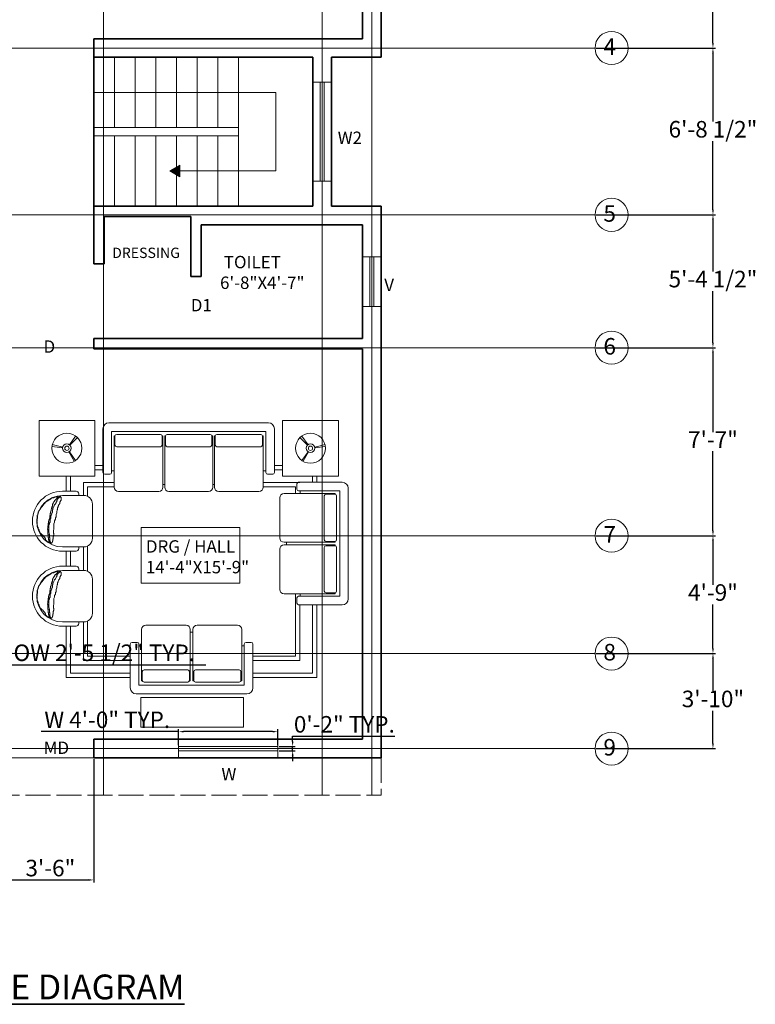
# Model space of a CAD drawing. Units: inches. Extents: x 1070 to 2371, y 645 to 1546.
# Tile 9 of 10: x 2015 to 2371, y 686 to 1162. Entities that reach past the tile are written whole.
import ezdxf

# ---------------------------------------------------------------- set-up
doc = ezdxf.new("R2010")
doc.units = ezdxf.units.IN
doc.linetypes.add('ACAD_ISO02W100', pattern=[15, 12, -3])
for name, color, linetype, lineweight in [('A-ANNO-DIMS', 2, 'Continuous', 18), ('A-ANNO-SYMB', 7, 'Continuous', 18), ('A-ANNO-TEXT', 7, 'Continuous', 18), ('A-ANNO-TITL', 7, 'Continuous', 35), ('A-AREA-IDEN', 7, 'Continuous', 18), ('A-DOOR', 4, 'Continuous', 18), ('A-FLOR-STRS', 7, 'Continuous', 18), ('A-FURN', 8, 'Continuous', 18), ('A-GLAZ', 4, 'Continuous', 18), ('A-GRID', 8, 'Continuous', 13), ('A-GRID-IDEN', 7, 'Continuous', 18), ('A-ROOF-OVHD', 8, 'ACAD_ISO02W100', 13), ('A-WALL', 7, 'Continuous', 35)]:
    doc.layers.add(name, color=color, linetype=linetype, lineweight=lineweight)
doc.styles.get("Standard").update_dxf_attribs({"font": 'arial.ttf'})
doc.dimstyles.new('ISO-25', dxfattribs={"dimtxt": 8, "dimasz": 2.5, "dimexe": 1.25, "dimexo": 0.625, "dimtad": 1, "dimtih": 1, "dimtoh": 1, "dimdec": 1, "dimlunit": 3, "dimtxsty": 'Standard', "dimcen": 2.5, "dimadec": 0, "dimazin": 0, "dimtfac": 1, "dimtdec": 1, "dimtmove": 0, "dimatfit": 3, "dimfxl": 1, "dimarcsym": 0})

# ---------------------------------------------------------------- blocks, each defined once
blk = doc.blocks.new('A$C71DE5BFE')
for p, q in [((823, 3482), (823, 2972)), ((2753, 3552), (893, 3552)), ((923, 3452), (2723, 3452)), ((923, 2972), (923, 3452)), ((2723, 3452), (2723, 2972)), ((2823, 2972), (2823, 3482)), ((431, 3296), (503, 3397)), ((437, 3290), (525, 3379)), ((963, 3400), (953, 3400)), ((953, 3400), (953, 2802)), ((963, 3292), (963, 3396)), ((1493, 3416), (983, 3416)), ((1523, 3400), (1513, 3400)), ((1513, 3292), (1513, 3396)), ((1523, 2802), (1523, 3400)), ((1553, 3400), (1543, 3400)), ((1543, 2802), (1543, 3400)), ((1553, 3292), (1553, 3396)), ((2073, 3416), (1573, 3416)), ((2103, 3400), (2093, 3400)), ((2093, 3292), (2093, 3396)), ((2103, 2802), (2103, 3400)), ((2133, 3400), (2123, 3400)), ((2123, 2802), (2123, 3400)), ((2133, 3292), (2133, 3396)), ((2663, 3416), (2153, 3416)), ((2693, 3400), (2683, 3400)), ((2683, 3292), (2683, 3396)), ((2693, 2802), (2693, 3400)), ((3209, 3290), (3121, 3379)), ((3215, 3296), (3143, 3397)), ((352, 3261), (228, 3277)), ((353, 3267), (232, 3297)), ((1493, 3272), (983, 3272)), ((2073, 3272), (1573, 3272)), ((2663, 3272), (2153, 3272)), ((3293, 3267), (3414, 3297)), ((3294, 3261), (3418, 3277)), ((426, 3212), (488, 3103)), ((431, 3214), (503, 3113)), ((3215, 3214), (3143, 3113)), ((3220, 3212), (3158, 3103)), ((727, 3055), (823, 3055)), ((727, 3005), (823, 3005)), ((953, 2992), (923, 2992)), ((2723, 2992), (2693, 2992)), ((2823, 3055), (2919, 3055)), ((2823, 3005), (2919, 3005)), ((394, 2754), (394, 2930)), ((444, 2754), (444, 2930)), ((843, 2952), (903, 2952)), ((2743, 2952), (2803, 2952)), ((3269, 2930), (3269, 2858)), ((3319, 2930), (3319, 2858)), ((1543, 2832), (1523, 2832)), ((2123, 2832), (2103, 2832)), ((2693, 2855), (3119, 2855)), ((2693, 2805), (3069, 2805)), ((3069, 2805), (3069, 2728)), ((3085, 2838), (3085, 2778)), ((3615, 2858), (3105, 2858)), ((3105, 2758), (3585, 2758)), ((3125, 2728), (3125, 2758)), ((3585, 2758), (3585, 1528)), ((3685, 1498), (3685, 2788)), ((180, 2642), (185, 2647)), ((185, 2647), (189, 2649)), ((189, 2649), (193, 2651)), ((193, 2651), (198, 2653)), ((198, 2653), (202, 2655)), ((202, 2655), (206, 2660)), ((206, 2660), (211, 2662)), ((211, 2662), (213, 2666)), ((213, 2666), (217, 2669)), ((217, 2669), (220, 2673)), ((220, 2673), (224, 2673)), ((224, 2673), (228, 2675)), ((228, 2675), (233, 2677)), ((233, 2677), (246, 2677)), ((246, 2677), (250, 2679)), ((250, 2679), (255, 2682)), ((255, 2682), (257, 2686)), ((257, 2686), (261, 2686)), ((259, 2642), (261, 2647)), ((261, 2686), (266, 2688)), ((261, 2647), (263, 2651)), ((263, 2651), (268, 2655)), ((266, 2688), (270, 2688)), ((268, 2655), (272, 2658)), ((270, 2688), (274, 2690)), ((272, 2658), (276, 2662)), ((274, 2690), (283, 2690)), ((276, 2662), (281, 2664)), ((281, 2664), (283, 2669)), ((283, 2690), (288, 2692)), ((283, 2669), (285, 2673)), ((285, 2673), (290, 2677)), ((288, 2649), (285, 2644)), ((285, 2644), (285, 2638)), ((288, 2692), (305, 2692)), ((290, 2655), (288, 2649)), ((290, 2677), (292, 2682)), ((292, 2660), (290, 2655)), ((292, 2682), (296, 2686)), ((296, 2664), (292, 2660)), ((296, 2686), (299, 2690)), ((301, 2669), (296, 2664)), ((299, 2690), (301, 2695)), ((301, 2695), (303, 2695)), ((305, 2675), (301, 2669)), ((305, 2692), (310, 2695)), ((310, 2677), (305, 2675)), ((310, 2695), (323, 2695)), ((312, 2682), (310, 2677)), ((316, 2684), (312, 2682)), ((321, 2686), (316, 2684)), ((318, 2697), (323, 2697)), ((323, 2690), (321, 2686)), ((323, 2695), (327, 2697)), ((323, 2697), (327, 2695)), ((327, 2695), (323, 2690)), ((327, 2697), (329, 2697)), ((327, 2695), (331, 2686)), ((331, 2647), (329, 2642)), ((331, 2686), (334, 2682)), ((334, 2651), (331, 2647)), ((334, 2682), (334, 2677)), ((334, 2677), (336, 2673)), ((336, 2660), (334, 2655)), ((334, 2655), (334, 2651)), ((336, 2673), (336, 2660)), ((350, 2754), (510, 2754)), ((350, 2704), (600, 2704)), ((540, 2724), (540, 2704)), ((1473, 2752), (1003, 2752)), ((2053, 2752), (1593, 2752)), ((2643, 2752), (2173, 2752)), ((2885, 2208), (2885, 2678)), ((3533, 2728), (2935, 2728)), ((3405, 2188), (3405, 2698)), ((3425, 2718), (3529, 2718)), ((3533, 2717), (3533, 2728)), ((3549, 2188), (3549, 2698)), ((75, 2524), (79, 2528)), ((79, 2528), (84, 2530)), ((84, 2530), (86, 2535)), ((86, 2535), (88, 2539)), ((88, 2539), (90, 2544)), ((90, 2544), (93, 2548)), ((93, 2548), (95, 2552)), ((95, 2552), (99, 2557)), ((99, 2561), (104, 2563)), ((99, 2557), (99, 2561)), ((104, 2563), (106, 2568)), ((106, 2568), (110, 2568)), ((110, 2572), (114, 2574)), ((110, 2568), (110, 2572)), ((114, 2574), (117, 2579)), ((117, 2579), (119, 2583)), ((119, 2583), (123, 2585)), ((123, 2589), (127, 2592)), ((123, 2585), (123, 2589)), ((127, 2592), (130, 2596)), ((130, 2596), (134, 2600)), ((134, 2600), (136, 2605)), ((136, 2605), (138, 2609)), ((138, 2609), (143, 2611)), ((143, 2616), (147, 2618)), ((143, 2611), (143, 2616)), ((147, 2618), (149, 2622)), ((149, 2622), (154, 2625)), ((154, 2625), (158, 2627)), ((158, 2627), (163, 2631)), ((163, 2631), (167, 2636)), ((167, 2636), (171, 2638)), ((171, 2638), (176, 2640)), ((176, 2640), (180, 2642)), ((217, 2530), (220, 2535)), ((217, 2526), (217, 2530)), ((220, 2541), (222, 2548)), ((220, 2535), (220, 2541)), ((222, 2552), (224, 2557)), ((222, 2548), (222, 2552)), ((224, 2557), (226, 2561)), ((226, 2561), (228, 2566)), ((228, 2566), (231, 2570)), ((231, 2574), (233, 2581)), ((231, 2570), (231, 2574)), ((233, 2589), (235, 2594)), ((233, 2581), (233, 2589)), ((235, 2535), (233, 2530)), ((233, 2530), (233, 2511)), ((235, 2598), (237, 2603)), ((235, 2594), (235, 2598)), ((237, 2541), (235, 2535)), ((237, 2603), (239, 2607)), ((239, 2552), (237, 2546)), ((237, 2546), (237, 2541)), ((239, 2611), (242, 2616)), ((239, 2607), (239, 2611)), ((242, 2561), (239, 2557)), ((239, 2557), (239, 2552)), ((242, 2616), (244, 2620)), ((244, 2568), (242, 2561)), ((244, 2620), (248, 2625)), ((248, 2574), (244, 2568)), ((248, 2625), (250, 2629)), ((250, 2579), (248, 2574)), ((250, 2629), (253, 2633)), ((255, 2585), (250, 2579)), ((253, 2633), (257, 2638)), ((259, 2594), (255, 2585)), ((257, 2638), (259, 2642)), ((268, 2605), (259, 2594)), ((272, 2616), (268, 2605)), ((276, 2620), (272, 2616)), ((281, 2629), (276, 2625)), ((276, 2625), (276, 2620)), ((283, 2633), (281, 2629)), ((285, 2638), (283, 2633)), ((290, 2528), (285, 2519)), ((292, 2541), (290, 2535)), ((290, 2535), (290, 2528)), ((294, 2557), (292, 2548)), ((292, 2548), (292, 2541)), ((299, 2570), (294, 2561)), ((294, 2561), (294, 2557)), ((301, 2579), (299, 2570)), ((303, 2585), (301, 2579)), ((312, 2598), (303, 2589)), ((303, 2589), (303, 2585)), ((316, 2607), (312, 2598)), ((318, 2611), (316, 2607)), ((321, 2620), (318, 2616)), ((318, 2616), (318, 2611)), ((323, 2629), (321, 2625)), ((321, 2625), (321, 2620)), ((325, 2633), (323, 2629)), ((329, 2638), (325, 2633)), ((329, 2642), (329, 2638)), ((700, 2604), (700, 2204)), ((55, 2423), (57, 2427)), ((55, 2405), (55, 2423)), ((57, 2471), (60, 2476)), ((57, 2463), (57, 2471)), ((60, 2458), (57, 2463)), ((57, 2436), (60, 2441)), ((57, 2427), (57, 2436)), ((60, 2476), (62, 2480)), ((60, 2441), (60, 2458)), ((62, 2480), (64, 2484)), ((64, 2489), (66, 2493)), ((64, 2484), (64, 2489)), ((66, 2497), (68, 2502)), ((66, 2493), (66, 2497)), ((68, 2511), (71, 2515)), ((68, 2502), (68, 2511)), ((71, 2515), (73, 2519)), ((73, 2519), (75, 2524)), ((191, 2405), (193, 2414)), ((193, 2414), (198, 2427)), ((198, 2427), (200, 2432)), ((200, 2432), (202, 2436)), ((202, 2441), (204, 2445)), ((202, 2436), (202, 2441)), ((204, 2465), (206, 2469)), ((204, 2445), (204, 2465)), ((206, 2493), (209, 2497)), ((206, 2469), (206, 2493)), ((215, 2436), (206, 2419)), ((206, 2419), (206, 2392)), ((209, 2506), (211, 2511)), ((209, 2497), (209, 2506)), ((211, 2515), (213, 2519)), ((211, 2511), (211, 2515)), ((213, 2519), (217, 2526)), ((217, 2471), (215, 2467)), ((215, 2467), (215, 2436)), ((220, 2476), (217, 2471)), ((222, 2482), (220, 2476)), ((224, 2487), (222, 2482)), ((226, 2491), (224, 2487)), ((228, 2497), (226, 2491)), ((231, 2504), (228, 2497)), ((233, 2511), (231, 2504)), ((268, 2427), (259, 2410)), ((276, 2454), (268, 2445)), ((268, 2445), (268, 2427)), ((285, 2500), (276, 2482)), ((276, 2482), (276, 2454)), ((285, 2519), (285, 2500)), ((53, 2401), (55, 2405)), ((53, 2392), (53, 2401)), ((55, 2388), (53, 2392)), ((55, 2362), (55, 2388)), ((57, 2357), (55, 2362)), ((57, 2353), (57, 2357)), ((60, 2349), (57, 2353)), ((60, 2344), (60, 2349)), ((62, 2340), (60, 2344)), ((64, 2335), (62, 2340)), ((66, 2331), (64, 2335)), ((66, 2327), (66, 2331)), ((68, 2322), (66, 2327)), ((68, 2318), (68, 2322)), ((71, 2311), (68, 2318)), ((73, 2307), (71, 2311)), ((75, 2302), (73, 2307)), ((77, 2298), (75, 2302)), ((77, 2294), (77, 2298)), ((176, 2316), (178, 2322)), ((176, 2311), (176, 2316)), ((178, 2307), (176, 2311)), ((178, 2335), (180, 2342)), ((178, 2322), (178, 2335)), ((178, 2298), (178, 2307)), ((180, 2294), (178, 2298)), ((180, 2351), (183, 2357)), ((180, 2342), (180, 2351)), ((183, 2357), (185, 2364)), ((185, 2377), (187, 2381)), ((185, 2364), (185, 2377)), ((187, 2392), (189, 2397)), ((187, 2381), (187, 2392)), ((189, 2401), (191, 2405)), ((189, 2397), (189, 2401)), ((195, 2364), (193, 2360)), ((193, 2360), (193, 2274)), ((198, 2373), (195, 2368)), ((195, 2368), (195, 2364)), ((206, 2392), (198, 2384)), ((198, 2384), (198, 2373)), ((248, 2307), (246, 2300)), ((246, 2300), (246, 2263)), ((250, 2371), (248, 2366)), ((248, 2366), (248, 2307)), ((259, 2392), (250, 2375)), ((250, 2375), (250, 2371)), ((259, 2410), (259, 2392)), ((79, 2289), (77, 2294)), ((82, 2285), (79, 2289)), ((84, 2279), (82, 2285)), ((86, 2274), (84, 2279)), ((88, 2270), (86, 2274)), ((90, 2265), (88, 2270)), ((95, 2263), (90, 2265)), ((97, 2259), (95, 2263)), ((101, 2257), (97, 2259)), ((104, 2252), (101, 2257)), ((108, 2250), (104, 2252)), ((112, 2246), (108, 2250)), ((121, 2239), (112, 2246)), ((134, 2226), (121, 2239)), ((136, 2221), (134, 2226)), ((141, 2219), (136, 2221)), ((143, 2215), (141, 2219)), ((145, 2210), (143, 2215)), ((147, 2206), (145, 2210)), ((149, 2202), (147, 2206)), ((152, 2197), (149, 2202)), ((154, 2191), (152, 2197)), ((154, 2186), (154, 2191)), ((156, 2182), (154, 2186)), ((180, 2254), (180, 2294)), ((183, 2250), (180, 2254)), ((183, 2246), (183, 2250)), ((185, 2239), (183, 2246)), ((185, 2213), (185, 2239)), ((187, 2208), (185, 2213)), ((187, 2204), (187, 2208)), ((189, 2199), (187, 2204)), ((189, 2191), (189, 2199)), ((191, 2186), (189, 2191)), ((191, 2180), (191, 2186)), ((193, 2274), (195, 2265)), ((195, 2265), (195, 2252)), ((195, 2252), (198, 2248)), ((198, 2248), (198, 2243)), ((198, 2243), (200, 2232)), ((200, 2232), (200, 2215)), ((200, 2215), (202, 2208)), ((202, 2208), (202, 2186)), ((202, 2186), (204, 2182)), ((239, 2184), (237, 2180)), ((242, 2197), (239, 2193)), ((239, 2193), (239, 2184)), ((244, 2228), (242, 2224)), ((242, 2224), (242, 2197)), ((246, 2237), (244, 2232)), ((244, 2232), (244, 2228)), ((246, 2263), (248, 2259)), ((248, 2241), (246, 2237)), ((248, 2259), (248, 2241)), ((160, 2180), (156, 2182)), ((163, 2176), (160, 2180)), ((167, 2171), (163, 2176)), ((169, 2167), (167, 2171)), ((174, 2167), (169, 2167)), ((176, 2162), (174, 2167)), ((180, 2162), (176, 2162)), ((185, 2160), (180, 2162)), ((189, 2158), (185, 2160)), ((195, 2154), (189, 2158)), ((193, 2176), (191, 2180)), ((195, 2171), (193, 2176)), ((195, 2162), (195, 2171)), ((198, 2158), (195, 2162)), ((200, 2151), (195, 2154)), ((200, 2154), (198, 2158)), ((200, 2149), (200, 2154)), ((204, 2149), (200, 2151)), ((204, 2182), (204, 2173)), ((204, 2173), (206, 2169)), ((209, 2147), (204, 2149)), ((206, 2169), (206, 2165)), ((206, 2165), (209, 2160)), ((209, 2160), (211, 2156)), ((213, 2149), (209, 2147)), ((211, 2156), (213, 2151)), ((213, 2151), (213, 2149)), ((226, 2149), (213, 2149)), ((228, 2154), (226, 2149)), ((233, 2158), (228, 2154)), ((235, 2162), (233, 2158)), ((237, 2176), (235, 2171)), ((235, 2171), (235, 2162)), ((237, 2180), (237, 2176)), ((350, 2104), (600, 2104)), ((540, 2104), (540, 2084)), ((594, 1829), (594, 2104)), ((644, 1819), (644, 2114)), ((2885, 1608), (2885, 2078)), ((2935, 2158), (3533, 2158)), ((2935, 2128), (3533, 2128)), ((2965, 2138), (2965, 2158)), ((2965, 2128), (2965, 2148)), ((3405, 1588), (3405, 2098)), ((3425, 2168), (3529, 2168)), ((3425, 2118), (3529, 2118)), ((3533, 2158), (3533, 2168)), ((3533, 2117), (3533, 2128)), ((3549, 1588), (3549, 2098)), ((510, 2054), (350, 2054)), ((394, 1879), (394, 2054)), ((444, 1879), (444, 2054)), ((350, 1879), (510, 1879)), ((540, 1849), (540, 1829)), ((130, 1721), (134, 1725)), ((134, 1725), (136, 1730)), ((136, 1730), (138, 1734)), ((138, 1734), (143, 1736)), ((143, 1741), (147, 1743)), ((143, 1736), (143, 1741)), ((147, 1743), (149, 1747)), ((149, 1747), (154, 1750)), ((154, 1750), (158, 1752)), ((158, 1752), (163, 1756)), ((163, 1756), (167, 1761)), ((167, 1761), (171, 1763)), ((171, 1763), (176, 1765)), ((176, 1765), (180, 1767)), ((180, 1767), (185, 1772)), ((185, 1772), (189, 1774)), ((189, 1774), (193, 1776)), ((193, 1776), (198, 1778)), ((198, 1778), (202, 1780)), ((202, 1780), (206, 1785)), ((206, 1785), (211, 1787)), ((211, 1787), (213, 1791)), ((213, 1791), (217, 1794)), ((217, 1794), (220, 1798)), ((220, 1798), (224, 1798)), ((224, 1798), (228, 1800)), ((228, 1800), (233, 1802)), ((233, 1802), (246, 1802)), ((235, 1723), (237, 1728)), ((237, 1728), (239, 1732)), ((239, 1736), (242, 1741)), ((239, 1732), (239, 1736)), ((242, 1741), (244, 1745)), ((244, 1745), (248, 1750)), ((246, 1802), (250, 1804)), ((248, 1750), (250, 1754)), ((250, 1804), (255, 1807)), ((250, 1754), (253, 1758)), ((253, 1758), (257, 1763)), ((255, 1807), (257, 1811)), ((257, 1811), (261, 1811)), ((257, 1763), (259, 1767)), ((259, 1767), (261, 1772)), ((268, 1730), (259, 1719)), ((261, 1811), (266, 1813)), ((261, 1772), (263, 1776)), ((263, 1776), (268, 1780)), ((266, 1813), (270, 1813)), ((268, 1780), (272, 1783)), ((272, 1741), (268, 1730)), ((270, 1813), (274, 1815)), ((272, 1783), (276, 1787)), ((276, 1745), (272, 1741)), ((274, 1815), (283, 1815)), ((276, 1787), (281, 1789)), ((281, 1754), (276, 1750)), ((276, 1750), (276, 1745)), ((281, 1789), (283, 1794)), ((283, 1758), (281, 1754)), ((283, 1815), (288, 1817)), ((283, 1794), (285, 1798)), ((285, 1763), (283, 1758)), ((285, 1798), (290, 1802)), ((288, 1774), (285, 1769)), ((285, 1769), (285, 1763)), ((288, 1817), (305, 1817)), ((290, 1780), (288, 1774)), ((290, 1802), (292, 1807)), ((292, 1785), (290, 1780)), ((292, 1807), (296, 1811)), ((296, 1789), (292, 1785)), ((296, 1811), (299, 1815)), ((301, 1794), (296, 1789)), ((299, 1815), (301, 1820)), ((301, 1820), (303, 1820)), ((305, 1800), (301, 1794)), ((305, 1817), (310, 1820)), ((310, 1802), (305, 1800)), ((310, 1820), (323, 1820)), ((312, 1807), (310, 1802)), ((316, 1809), (312, 1807)), ((316, 1732), (312, 1723)), ((321, 1811), (316, 1809)), ((318, 1736), (316, 1732)), ((318, 1822), (323, 1822)), ((321, 1745), (318, 1741)), ((318, 1741), (318, 1736)), ((323, 1815), (321, 1811)), ((323, 1754), (321, 1750)), ((321, 1750), (321, 1745)), ((323, 1820), (327, 1822)), ((323, 1822), (327, 1820)), ((327, 1820), (323, 1815)), ((325, 1758), (323, 1754)), ((329, 1763), (325, 1758)), ((327, 1822), (329, 1822)), ((327, 1820), (331, 1811)), ((331, 1772), (329, 1767)), ((329, 1767), (329, 1763)), ((331, 1811), (334, 1807)), ((334, 1776), (331, 1772)), ((334, 1807), (334, 1802)), ((334, 1802), (336, 1798)), ((336, 1785), (334, 1780)), ((334, 1780), (334, 1776)), ((336, 1798), (336, 1785)), ((350, 1829), (600, 1829)), ((700, 1729), (700, 1329)), ((62, 1605), (64, 1609)), ((64, 1614), (66, 1618)), ((64, 1609), (64, 1614)), ((66, 1622), (68, 1627)), ((66, 1618), (66, 1622)), ((68, 1636), (71, 1640)), ((68, 1627), (68, 1636)), ((71, 1640), (73, 1644)), ((73, 1644), (75, 1649)), ((75, 1649), (79, 1653)), ((79, 1653), (84, 1655)), ((84, 1655), (86, 1660)), ((86, 1660), (88, 1664)), ((88, 1664), (90, 1669)), ((90, 1669), (93, 1673)), ((93, 1673), (95, 1677)), ((95, 1677), (99, 1682)), ((99, 1686), (104, 1688)), ((99, 1682), (99, 1686)), ((104, 1688), (106, 1693)), ((106, 1693), (110, 1693)), ((110, 1697), (114, 1699)), ((110, 1693), (110, 1697)), ((114, 1699), (117, 1704)), ((117, 1704), (119, 1708)), ((119, 1708), (123, 1710)), ((123, 1714), (127, 1717)), ((123, 1710), (123, 1714)), ((127, 1717), (130, 1721)), ((206, 1618), (209, 1622)), ((206, 1594), (206, 1618)), ((209, 1631), (211, 1636)), ((209, 1622), (209, 1631)), ((211, 1640), (213, 1644)), ((211, 1636), (211, 1640)), ((213, 1644), (217, 1651)), ((217, 1655), (220, 1660)), ((217, 1651), (217, 1655)), ((220, 1666), (222, 1673)), ((220, 1660), (220, 1666)), ((222, 1677), (224, 1682)), ((222, 1673), (222, 1677)), ((224, 1612), (222, 1607)), ((224, 1682), (226, 1686)), ((226, 1616), (224, 1612)), ((226, 1686), (228, 1691)), ((228, 1622), (226, 1616)), ((228, 1691), (231, 1695)), ((231, 1629), (228, 1622)), ((231, 1699), (233, 1706)), ((231, 1695), (231, 1699)), ((233, 1636), (231, 1629)), ((233, 1714), (235, 1719)), ((233, 1706), (233, 1714)), ((235, 1660), (233, 1655)), ((233, 1655), (233, 1636)), ((235, 1719), (235, 1723)), ((237, 1666), (235, 1660)), ((239, 1677), (237, 1671)), ((237, 1671), (237, 1666)), ((242, 1686), (239, 1682)), ((239, 1682), (239, 1677)), ((244, 1693), (242, 1686)), ((248, 1699), (244, 1693)), ((250, 1704), (248, 1699)), ((255, 1710), (250, 1704)), ((259, 1719), (255, 1710)), ((285, 1625), (276, 1607)), ((290, 1653), (285, 1644)), ((285, 1644), (285, 1625)), ((292, 1666), (290, 1660)), ((290, 1660), (290, 1653)), ((294, 1682), (292, 1673)), ((292, 1673), (292, 1666)), ((299, 1695), (294, 1686)), ((294, 1686), (294, 1682)), ((301, 1704), (299, 1695)), ((303, 1710), (301, 1704)), ((312, 1723), (303, 1714)), ((303, 1714), (303, 1710)), ((53, 1526), (55, 1530)), ((53, 1517), (53, 1526)), ((55, 1513), (53, 1517)), ((55, 1548), (57, 1552)), ((55, 1530), (55, 1548)), ((55, 1487), (55, 1513)), ((57, 1596), (60, 1601)), ((57, 1588), (57, 1596)), ((60, 1583), (57, 1588)), ((57, 1561), (60, 1566)), ((57, 1552), (57, 1561)), ((60, 1601), (62, 1605)), ((60, 1566), (60, 1583)), ((185, 1502), (187, 1506)), ((185, 1489), (185, 1502)), ((187, 1517), (189, 1522)), ((187, 1506), (187, 1517)), ((189, 1526), (191, 1530)), ((189, 1522), (189, 1526)), ((191, 1530), (193, 1539)), ((193, 1539), (198, 1552)), ((198, 1498), (195, 1493)), ((198, 1552), (200, 1557)), ((206, 1517), (198, 1509)), ((198, 1509), (198, 1498)), ((200, 1557), (202, 1561)), ((202, 1566), (204, 1570)), ((202, 1561), (202, 1566)), ((204, 1590), (206, 1594)), ((204, 1570), (204, 1590)), ((215, 1561), (206, 1544)), ((206, 1544), (206, 1517)), ((217, 1596), (215, 1592)), ((215, 1592), (215, 1561)), ((220, 1601), (217, 1596)), ((222, 1607), (220, 1601)), ((250, 1496), (248, 1491)), ((259, 1517), (250, 1500)), ((250, 1500), (250, 1496)), ((268, 1552), (259, 1535)), ((259, 1535), (259, 1517)), ((276, 1579), (268, 1570)), ((268, 1570), (268, 1552)), ((276, 1607), (276, 1579)), ((2935, 1558), (3533, 1558)), ((3085, 1508), (3085, 1448)), ((3585, 1528), (3105, 1528)), ((3125, 1528), (3125, 1558)), ((3425, 1568), (3529, 1568)), ((3533, 1558), (3533, 1568)), ((57, 1482), (55, 1487)), ((57, 1478), (57, 1482)), ((60, 1474), (57, 1478)), ((60, 1469), (60, 1474)), ((62, 1465), (60, 1469)), ((64, 1460), (62, 1465)), ((66, 1456), (64, 1460)), ((66, 1452), (66, 1456)), ((68, 1447), (66, 1452)), ((68, 1443), (68, 1447)), ((71, 1436), (68, 1443)), ((73, 1432), (71, 1436)), ((75, 1427), (73, 1432)), ((77, 1423), (75, 1427)), ((77, 1419), (77, 1423)), ((79, 1414), (77, 1419)), ((82, 1410), (79, 1414)), ((84, 1404), (82, 1410)), ((86, 1399), (84, 1404)), ((88, 1395), (86, 1399)), ((90, 1390), (88, 1395)), ((95, 1388), (90, 1390)), ((97, 1384), (95, 1388)), ((101, 1382), (97, 1384)), ((104, 1377), (101, 1382)), ((176, 1441), (178, 1447)), ((176, 1436), (176, 1441)), ((178, 1432), (176, 1436)), ((178, 1460), (180, 1467)), ((178, 1447), (178, 1460)), ((178, 1423), (178, 1432)), ((180, 1419), (178, 1423)), ((180, 1476), (183, 1482)), ((180, 1467), (180, 1476)), ((180, 1379), (180, 1419)), ((183, 1375), (180, 1379)), ((183, 1482), (185, 1489)), ((195, 1489), (193, 1485)), ((193, 1485), (193, 1399)), ((193, 1399), (195, 1390)), ((195, 1493), (195, 1489)), ((195, 1390), (195, 1377)), ((248, 1432), (246, 1425)), ((246, 1425), (246, 1388)), ((246, 1388), (248, 1384)), ((248, 1491), (248, 1432)), ((248, 1384), (248, 1366)), ((3105, 1428), (3615, 1428)), ((108, 1375), (104, 1377)), ((112, 1371), (108, 1375)), ((121, 1364), (112, 1371)), ((134, 1351), (121, 1364)), ((136, 1346), (134, 1351)), ((141, 1344), (136, 1346)), ((143, 1340), (141, 1344)), ((145, 1335), (143, 1340)), ((147, 1331), (145, 1335)), ((149, 1327), (147, 1331)), ((152, 1322), (149, 1327)), ((154, 1316), (152, 1322)), ((154, 1311), (154, 1316)), ((156, 1307), (154, 1311)), ((160, 1305), (156, 1307)), ((163, 1301), (160, 1305)), ((167, 1296), (163, 1301)), ((169, 1292), (167, 1296)), ((174, 1292), (169, 1292)), ((176, 1287), (174, 1292)), ((180, 1287), (176, 1287)), ((185, 1285), (180, 1287)), ((183, 1371), (183, 1375)), ((185, 1364), (183, 1371)), ((185, 1338), (185, 1364)), ((187, 1333), (185, 1338)), ((189, 1283), (185, 1285)), ((187, 1329), (187, 1333)), ((189, 1324), (187, 1329)), ((189, 1316), (189, 1324)), ((191, 1311), (189, 1316)), ((195, 1279), (189, 1283)), ((191, 1305), (191, 1311)), ((193, 1301), (191, 1305)), ((195, 1296), (193, 1301)), ((195, 1377), (198, 1373)), ((195, 1287), (195, 1296)), ((198, 1283), (195, 1287)), ((200, 1276), (195, 1279)), ((198, 1373), (198, 1368)), ((198, 1368), (200, 1357)), ((200, 1279), (198, 1283)), ((200, 1357), (200, 1340)), ((200, 1340), (202, 1333)), ((200, 1274), (200, 1279)), ((204, 1274), (200, 1276)), ((202, 1333), (202, 1311)), ((202, 1311), (204, 1307)), ((204, 1307), (204, 1298)), ((204, 1298), (206, 1294)), ((209, 1272), (204, 1274)), ((206, 1294), (206, 1290)), ((206, 1290), (209, 1285)), ((209, 1285), (211, 1281)), ((213, 1274), (209, 1272)), ((211, 1281), (213, 1276)), ((213, 1276), (213, 1274)), ((226, 1274), (213, 1274)), ((228, 1279), (226, 1274)), ((233, 1283), (228, 1279)), ((235, 1287), (233, 1283)), ((237, 1301), (235, 1296)), ((235, 1296), (235, 1287)), ((239, 1309), (237, 1305)), ((237, 1305), (237, 1301)), ((242, 1322), (239, 1318)), ((239, 1318), (239, 1309)), ((244, 1353), (242, 1349)), ((242, 1349), (242, 1322)), ((246, 1362), (244, 1357)), ((244, 1357), (244, 1353)), ((248, 1366), (246, 1362)), ((350, 1229), (600, 1229)), ((510, 1179), (350, 1179)), ((540, 1229), (540, 1209)), ((1322, 1189), (1792, 1189)), ((1922, 1189), (2392, 1189)), ((1272, 1139), (1272, 541)), ((1842, 1139), (1842, 541)), ((1842, 1109), (1862, 1109)), ((1852, 1109), (1872, 1109)), ((1872, 1139), (1872, 541)), ((2442, 541), (2442, 1139)), ((1142, 969), (1142, 459)), ((1222, 989), (1162, 989)), ((1242, 489), (1242, 969)), ((1242, 949), (1272, 949)), ((2442, 949), (2472, 949)), ((2472, 969), (2472, 489)), ((2552, 989), (2492, 989)), ((2572, 459), (2572, 969)), ((1282, 649), (1282, 546)), ((1302, 669), (1812, 669)), ((1832, 649), (1832, 546)), ((1882, 649), (1882, 546)), ((1902, 669), (2412, 669)), ((2432, 649), (2432, 546)), ((2472, 489), (1242, 489)), ((1272, 541), (1282, 541)), ((1302, 526), (1812, 526)), ((1832, 541), (1842, 541)), ((1872, 541), (1883, 541)), ((1902, 526), (2412, 526)), ((2432, 541), (2442, 541)), ((1212, 389), (2502, 389))]:
    blk.add_line(p, q)
for points in [[(727, 2930), (77, 2930), (77, 3580), (727, 3580)], [(2919, 2930), (3569, 2930), (3569, 3580), (2919, 3580)], [(2419, 1680), (2419, 2330), (1269, 2330), (1269, 1680)], [(2464, 0), (2464, 345), (1264, 345), (1264, 0)]]:
    blk.add_lwpolyline(points, close=True)
for points in [[(594, 2704), (594, 2855), (953, 2855)], [(644, 2694), (644, 2805), (953, 2805)], [(3069, 1558), (3069, 830), (2572, 830)], [(3269, 1428), (3269, 630), (2572, 630)], [(3319, 1428), (3319, 580), (2572, 580)], [(3119, 1428), (3119, 780), (2572, 780)], [(1142, 580), (394, 580), (394, 1179)], [(1142, 630), (444, 630), (444, 1179)], [(1142, 780), (594, 780), (594, 1229)], [(1142, 830), (644, 830), (644, 1239)]]:
    blk.add_lwpolyline(points)
for centre, radius in [((402, 3255), 175), ((3244, 3255), 175), ((402, 3255), 50), ((402, 3255), 25), ((3244, 3255), 50), ((3244, 3255), 25)]:
    blk.add_circle(centre, radius)
for centre, radius, start, end in [((893, 3482), 70, 90, 180), ((2753, 3482), 70, 0, 90), ((983, 3396), 20, 90, 180), ((1493, 3396), 20, 0, 90), ((1573, 3396), 20, 90, 180), ((2073, 3396), 20, 0, 90), ((2153, 3396), 20, 90, 180), ((2663, 3396), 20, 0, 90), ((983, 3292), 20, 180, 270), ((1493, 3292), 20, 270, 0), ((1573, 3292), 20, 180, 270), ((2073, 3292), 20, 270, 0), ((2153, 3292), 20, 180, 270), ((2663, 3292), 20, 270, 0), ((843, 2972), 20, 180, 270), ((903, 2972), 20, 270, 0), ((2743, 2972), 20, 180, 270), ((2803, 2972), 20, 270, 0), ((1003, 2802), 50, 180, 270), ((1473, 2802), 50, 270, 0), ((1593, 2802), 50, 180, 270), ((2053, 2802), 50, 270, 0), ((2173, 2802), 50, 180, 270), ((2643, 2802), 50, 270, 0), ((3105, 2838), 20, 90, 180), ((3105, 2778), 20, 180, 270), ((3615, 2788), 70, 0, 90), ((350, 2404), 350, 90, 270), ((350, 2404), 300, 90, 270), ((510, 2724), 30, 0, 90), ((600, 2604), 100, 0, 90), ((2935, 2678), 50, 90, 180), ((3425, 2698), 20, 90, 180), ((3529, 2698), 20, 0, 90), ((600, 2204), 100, 270, 0), ((2935, 2208), 50, 180, 270), ((3425, 2188), 20, 180, 270), ((3529, 2188), 20, 270, 0), ((510, 2084), 30, 270, 0), ((2935, 2078), 50, 90, 180), ((3425, 2098), 20, 90, 180), ((3529, 2098), 20, 0, 90), ((350, 1529), 350, 90, 270), ((510, 1849), 30, 0, 90), ((350, 1529), 300, 90, 270), ((600, 1729), 100, 0, 90), ((2935, 1608), 50, 180, 270), ((3105, 1508), 20, 90, 180), ((3425, 1588), 20, 180, 270), ((3529, 1588), 20, 270, 0), ((3615, 1498), 70, 270, 0), ((3105, 1448), 20, 180, 270), ((600, 1329), 100, 270, 0), ((510, 1209), 30, 270, 0), ((1322, 1139), 50, 90, 180), ((1792, 1139), 50, 0, 90), ((1922, 1139), 50, 90, 180), ((2392, 1139), 50, 0, 90), ((1162, 969), 20, 90, 180), ((1222, 969), 20, 0, 90), ((2492, 969), 20, 90, 180), ((2552, 969), 20, 0, 90), ((1302, 649), 20, 90, 180), ((1812, 649), 20, 0, 90), ((1902, 649), 20, 90, 180), ((2412, 649), 20, 0, 90), ((1302, 546), 20, 180, 270), ((1812, 546), 20, 270, 0), ((1902, 546), 20, 180, 270), ((2412, 546), 20, 270, 0), ((1212, 459), 70, 180, 270), ((2502, 459), 70, 270, 0)]:
    blk.add_arc(centre, radius, start, end)
blk = doc.blocks.new('GLAZ-48IN')
for p, q in [((0, 48), (0, 0)), ((2, 48), (2, 0))]:
    blk.add_line(p, q)
blk = doc.blocks.new('GLAZ-VENT-24IN')
for p, q in [((0, 2), (24, 2)), ((0, 0), (24, 0))]:
    blk.add_line(p, q)
blk = doc.blocks.new('STAIR-HALF-TURN')
for p, q in [((10, 72), (10, 38)), ((20, 72), (20, 38)), ((30, 72), (30, 38)), ((40, 72), (40, 38)), ((50, 72), (50, 38)), ((60, 72), (60, 38)), ((70, 72), (70, 0)), ((0, 38), (70, 38)), ((0, 34), (70, 34)), ((10, 34), (10, 0)), ((20, 34), (20, 0)), ((30, 34), (30, 0)), ((40, 34), (40, 18.86)), ((50, 34), (50, 0)), ((60, 34), (60, 0)), ((40, 15.14), (40, 0))]:
    blk.add_line(p, q)
blk = doc.blocks.new('STAIR-DIRECTION-RETURN')
h = blk.add_hatch(color=256)
h.dxf.hatch_style = 1
h.paths.add_polyline_path([(41.61, 5.58), (36.78, 2.79), (41.61, 0)])
for p, q in [((0, 40.79), (88.03, 40.79)), ((88.03, 40.79), (88.03, 2.79)), ((41.61, 2.79), (88.03, 2.79))]:
    blk.add_line(p, q)
blk.add_lwpolyline([(36.78, 2.79), (41.61, 0), (41.61, 5.58)], close=True)
blk = doc.blocks.new('*D25')
at = {"layer": 'A-ANNO-DIMS', "color": 0, "lineweight": -2, "transparency": 16777216}
for p, q in [((2091.54, 817.47), (2025.05, 817.47)), ((2091.54, 810.9), (2091.54, 818.72)), ((2137.04, 817.47), (2094.04, 817.47)), ((2139.54, 810.9), (2139.54, 818.72))]:
    blk.add_line(p, q, dxfattribs=at)
at = {"layer": 'A-ANNO-DIMS', "color": 0, "transparency": 16777216}
for points in [[(2094.04, 817.89), (2094.04, 817.06), (2091.54, 817.47)], [(2137.04, 817.89), (2137.04, 817.06), (2139.54, 817.47)]]:
    blk.add_solid(points, dxfattribs=at)
at = {"layer": 'Defpoints', "color": 0, "transparency": 16777216}
for p in [(2091.54, 817.47), (2091.54, 810.27), (2139.54, 810.27)]:
    blk.add_point(p, dxfattribs=at)
at = {"layer": 'A-ANNO-DIMS', "color": 0, "transparency": 16777216, "insert": (2057.05, 822.18), "char_height": 8, "attachment_point": 5}
blk.add_mtext('W 4\'-0" TYP.', dxfattribs=at)
blk = doc.blocks.new('*D26')
at = {"layer": 'A-ANNO-DIMS', "color": 0, "lineweight": -2, "transparency": 16777216}
for p, q in [((2146.74, 812.77), (2146.74, 815.27)), ((2146.74, 815.27), (2196.13, 815.27)), ((2140.17, 810.27), (2147.99, 810.27)), ((2146.74, 808.27), (2146.74, 810.27)), ((2140.17, 808.27), (2147.99, 808.27)), ((2146.74, 805.77), (2146.74, 803.27))]:
    blk.add_line(p, q, dxfattribs=at)
at = {"layer": 'A-ANNO-DIMS', "color": 0, "transparency": 16777216}
for points in [[(2146.33, 812.77), (2147.16, 812.77), (2146.74, 810.27)], [(2146.33, 805.77), (2147.16, 805.77), (2146.74, 808.27)]]:
    blk.add_solid(points, dxfattribs=at)
at = {"layer": 'Defpoints', "color": 0, "transparency": 16777216}
for p in [(2139.54, 810.27), (2146.74, 810.27), (2139.54, 808.27)]:
    blk.add_point(p, dxfattribs=at)
at = {"layer": 'A-ANNO-DIMS', "color": 0, "transparency": 16777216, "insert": (2171.75, 819.98), "char_height": 8, "attachment_point": 5}
blk.add_mtext('0\'-2" TYP.', dxfattribs=at)
blk = doc.blocks.new('*D37')
at = {"layer": 'A-ANNO-DIMS', "color": 0, "lineweight": -2, "transparency": 16777216}
for p, q in [((1900.54, 853.65), (1900.54, 848.6)), ((1930.04, 853.65), (1930.04, 848.6)), ((1903.04, 849.85), (1927.54, 849.85)), ((1930.04, 849.85), (2104.79, 849.85))]:
    blk.add_line(p, q, dxfattribs=at)
at = {"layer": 'A-ANNO-DIMS', "color": 0, "transparency": 16777216}
for points in [[(1903.04, 850.26), (1903.04, 849.43), (1900.54, 849.85)], [(1927.54, 850.26), (1927.54, 849.43), (1930.04, 849.85)]]:
    blk.add_solid(points, dxfattribs=at)
at = {"layer": 'Defpoints', "color": 0, "transparency": 16777216}
for p in [(1900.54, 854.27), (1930.04, 854.27), (1930.04, 849.85)]:
    blk.add_point(p, dxfattribs=at)
at = {"layer": 'A-ANNO-DIMS', "color": 0, "transparency": 16777216, "insert": (2018.67, 854.61), "char_height": 8, "attachment_point": 5}
blk.add_mtext('CORNER WINDOW 2\'-5 1/2" TYP.', dxfattribs=at)
blk = doc.blocks.new('*D51')
at = {"layer": 'A-ANNO-DIMS', "color": 0, "lineweight": -2, "transparency": 16777216}
for p, q in [((2008.54, 804.15), (2008.54, 744.47)), ((2050.54, 804.15), (2050.54, 744.47)), ((2011.04, 745.72), (2048.04, 745.72))]:
    blk.add_line(p, q, dxfattribs=at)
at = {"layer": 'A-ANNO-DIMS', "color": 0, "transparency": 16777216}
for points in [[(2011.04, 746.14), (2011.04, 745.31), (2008.54, 745.72)], [(2048.04, 746.14), (2048.04, 745.31), (2050.54, 745.72)]]:
    blk.add_solid(points, dxfattribs=at)
at = {"layer": 'Defpoints', "color": 0, "transparency": 16777216}
for p in [(2008.54, 804.77), (2050.54, 804.77), (2050.54, 745.72)]:
    blk.add_point(p, dxfattribs=at)
at = {"layer": 'A-ANNO-DIMS', "color": 0, "transparency": 16777216, "insert": (2029.54, 750.43), "char_height": 8, "attachment_point": 5}
blk.add_mtext('3\'-6"', dxfattribs=at)
blk = doc.blocks.new('*D63')
at = {"layer": 'A-ANNO-DIMS', "color": 0, "lineweight": -2, "transparency": 16777216}
for p, q in [((2293.65, 1194.27), (2351.32, 1194.27)), ((2350.07, 1191.77), (2350.07, 1175.98)), ((2350.07, 1150.77), (2350.07, 1166.56)), ((2293.65, 1148.27), (2351.32, 1148.27))]:
    blk.add_line(p, q, dxfattribs=at)
at = {"layer": 'A-ANNO-DIMS', "color": 0, "transparency": 16777216}
for points in [[(2349.66, 1191.77), (2350.49, 1191.77), (2350.07, 1194.27)], [(2349.66, 1150.77), (2350.49, 1150.77), (2350.07, 1148.27)]]:
    blk.add_solid(points, dxfattribs=at)
at = {"layer": 'Defpoints', "color": 0, "transparency": 16777216}
for p in [(2293.02, 1194.27), (2293.02, 1148.27), (2350.07, 1148.27)]:
    blk.add_point(p, dxfattribs=at)
at = {"layer": 'A-ANNO-DIMS', "color": 0, "transparency": 16777216, "insert": (2350.07, 1171.27), "char_height": 8, "attachment_point": 5}
blk.add_mtext('3\'-10"', dxfattribs=at)
blk = doc.blocks.new('*D64')
at = {"layer": 'A-ANNO-DIMS', "color": 0, "lineweight": -2, "transparency": 16777216}
for p, q in [((2293.65, 1148.27), (2351.32, 1148.27)), ((2350.07, 1145.77), (2350.07, 1112.68)), ((2350.07, 1070.06), (2350.07, 1103.16)), ((2293.65, 1067.56), (2351.32, 1067.56))]:
    blk.add_line(p, q, dxfattribs=at)
at = {"layer": 'A-ANNO-DIMS', "color": 0, "transparency": 16777216}
for points in [[(2349.66, 1145.77), (2350.49, 1145.77), (2350.07, 1148.27)], [(2349.66, 1070.06), (2350.49, 1070.06), (2350.07, 1067.56)]]:
    blk.add_solid(points, dxfattribs=at)
at = {"layer": 'Defpoints', "color": 0, "transparency": 16777216}
for p in [(2293.02, 1148.27), (2293.02, 1067.56), (2350.07, 1067.56)]:
    blk.add_point(p, dxfattribs=at)
at = {"layer": 'A-ANNO-DIMS', "color": 0, "transparency": 16777216, "insert": (2350.07, 1107.92), "char_height": 8, "attachment_point": 5}
blk.add_mtext('6\'-8 1/2"', dxfattribs=at)
blk = doc.blocks.new('*D65')
at = {"layer": 'A-ANNO-DIMS', "color": 0, "lineweight": -2, "transparency": 16777216}
for p, q in [((2293.65, 1067.56), (2351.32, 1067.56)), ((2350.07, 1065.06), (2350.07, 1040.18)), ((2350.07, 1005.77), (2350.07, 1030.66)), ((2293.65, 1003.27), (2351.32, 1003.27))]:
    blk.add_line(p, q, dxfattribs=at)
at = {"layer": 'A-ANNO-DIMS', "color": 0, "transparency": 16777216}
for points in [[(2349.66, 1065.06), (2350.49, 1065.06), (2350.07, 1067.56)], [(2349.66, 1005.77), (2350.49, 1005.77), (2350.07, 1003.27)]]:
    blk.add_solid(points, dxfattribs=at)
at = {"layer": 'Defpoints', "color": 0, "transparency": 16777216}
for p in [(2293.02, 1067.56), (2293.02, 1003.27), (2350.07, 1003.27)]:
    blk.add_point(p, dxfattribs=at)
at = {"layer": 'A-ANNO-DIMS', "color": 0, "transparency": 16777216, "insert": (2350.07, 1035.42), "char_height": 8, "attachment_point": 5}
blk.add_mtext('5\'-4 1/2"', dxfattribs=at)
blk = doc.blocks.new('*D66')
at = {"layer": 'A-ANNO-DIMS', "color": 0, "lineweight": -2, "transparency": 16777216}
for p, q in [((2293.65, 1003.27), (2351.32, 1003.27)), ((2350.07, 1000.77), (2350.07, 962.4)), ((2350.07, 914.77), (2350.07, 953.15)), ((2293.65, 912.27), (2351.32, 912.27))]:
    blk.add_line(p, q, dxfattribs=at)
at = {"layer": 'A-ANNO-DIMS', "color": 0, "transparency": 16777216}
for points in [[(2349.66, 1000.77), (2350.49, 1000.77), (2350.07, 1003.27)], [(2349.66, 914.77), (2350.49, 914.77), (2350.07, 912.27)]]:
    blk.add_solid(points, dxfattribs=at)
at = {"layer": 'Defpoints', "color": 0, "transparency": 16777216}
for p in [(2293.02, 1003.27), (2293.02, 912.27), (2350.07, 912.27)]:
    blk.add_point(p, dxfattribs=at)
at = {"layer": 'A-ANNO-DIMS', "color": 0, "transparency": 16777216, "insert": (2350.07, 957.77), "char_height": 8, "attachment_point": 5}
blk.add_mtext('7\'-7"', dxfattribs=at)
blk = doc.blocks.new('*D67')
at = {"layer": 'A-ANNO-DIMS', "color": 0, "lineweight": -2, "transparency": 16777216}
for p, q in [((2293.65, 912.27), (2351.32, 912.27)), ((2350.07, 909.77), (2350.07, 888.48)), ((2350.07, 857.77), (2350.07, 879.06)), ((2293.65, 855.27), (2351.32, 855.27))]:
    blk.add_line(p, q, dxfattribs=at)
at = {"layer": 'A-ANNO-DIMS', "color": 0, "transparency": 16777216}
for points in [[(2349.66, 909.77), (2350.49, 909.77), (2350.07, 912.27)], [(2349.66, 857.77), (2350.49, 857.77), (2350.07, 855.27)]]:
    blk.add_solid(points, dxfattribs=at)
at = {"layer": 'Defpoints', "color": 0, "transparency": 16777216}
for p in [(2293.02, 912.27), (2293.02, 855.27), (2350.07, 855.27)]:
    blk.add_point(p, dxfattribs=at)
at = {"layer": 'A-ANNO-DIMS', "color": 0, "transparency": 16777216, "insert": (2350.07, 883.77), "char_height": 8, "attachment_point": 5}
blk.add_mtext('4\'-9"', dxfattribs=at)
blk = doc.blocks.new('*D68')
at = {"layer": 'A-ANNO-DIMS', "color": 0, "lineweight": -2, "transparency": 16777216}
for p, q in [((2293.65, 855.27), (2351.32, 855.27)), ((2350.07, 852.77), (2350.07, 836.98)), ((2350.07, 811.77), (2350.07, 827.56)), ((2293.65, 809.27), (2351.32, 809.27))]:
    blk.add_line(p, q, dxfattribs=at)
at = {"layer": 'A-ANNO-DIMS', "color": 0, "transparency": 16777216}
for points in [[(2349.66, 852.77), (2350.49, 852.77), (2350.07, 855.27)], [(2349.66, 811.77), (2350.49, 811.77), (2350.07, 809.27)]]:
    blk.add_solid(points, dxfattribs=at)
at = {"layer": 'Defpoints', "color": 0, "transparency": 16777216}
for p in [(2293.02, 855.27), (2293.02, 809.27), (2350.07, 809.27)]:
    blk.add_point(p, dxfattribs=at)
at = {"layer": 'A-ANNO-DIMS', "color": 0, "transparency": 16777216, "insert": (2350.07, 832.27), "char_height": 8, "attachment_point": 5}
blk.add_mtext('3\'-10"', dxfattribs=at)

msp = doc.modelspace()

# ---------------------------------------------------------------- linework, layer by layer
at = {"layer": 'A-DOOR'}
msp.add_line((2008.54, 804.77), (2050.54, 804.77), dxfattribs=at)
at = {"layer": 'A-GLAZ'}
for p, q in [((2156.54, 1131.77), (2165.54, 1131.77)), ((2156.54, 1083.77), (2165.54, 1083.77)), ((2180.54, 1047.27), (2189.54, 1047.27)), ((2180.54, 1023.27), (2189.54, 1023.27)), ((2091.54, 813.77), (2091.54, 804.77)), ((2139.54, 813.77), (2139.54, 804.77))]:
    msp.add_line(p, q, dxfattribs=at)
at = {"layer": 'A-GRID'}
for p, q in [((2055.22, 786.77), (2055.22, 1478.99)), ((2161.04, 786.77), (2161.04, 1478.99)), ((2185.04, 786.77), (2185.04, 1478.99)), ((1795.54, 1148.27), (2293.02, 1148.27)), ((1795.54, 1067.56), (2293.02, 1067.56)), ((1777.54, 1003.27), (2293.02, 1003.27)), ((1777.54, 912.27), (2293.02, 912.27)), ((1777.54, 855.27), (2293.02, 855.27)), ((1999.54, 809.27), (2293.02, 809.27))]:
    msp.add_line(p, q, dxfattribs=at)
at = {"layer": 'A-GRID-IDEN'}
for centre in [(2301.02, 1148.27), (2301.02, 1067.56), (2301.02, 1003.27), (2301.02, 912.27), (2301.02, 855.27), (2301.02, 809.27)]:
    msp.add_circle(centre, 8, dxfattribs=at)
at = {"layer": 'A-ROOF-OVHD'}
for p in [(2189.54, 804.77), (1777.54, 786.77)]:
    msp.add_line(p, (2189.54, 786.77), dxfattribs=at)
at = {"layer": 'A-WALL'}
for p, q in [((2189.54, 1300.77), (2189.54, 1143.77)), ((2180.54, 1291.77), (2180.54, 1152.77)), ((2050.54, 1152.77), (2180.54, 1152.77)), ((2050.54, 1152.77), (2050.54, 1143.77)), ((2050.54, 1143.77), (2156.54, 1143.77)), ((2050.54, 1143.77), (2050.54, 1043.77)), ((2156.54, 1143.77), (2156.54, 1071.77)), ((2165.54, 1143.77), (2189.54, 1143.77)), ((2165.54, 1143.77), (2165.54, 1071.77)), ((2050.54, 1071.77), (2156.54, 1071.77)), ((2165.54, 1071.77), (2189.54, 1071.77)), ((2189.54, 1071.77), (2189.54, 804.77)), ((2055.54, 1066.77), (2097.54, 1066.77)), ((2055.54, 1066.77), (2055.54, 1043.77)), ((2097.54, 1066.77), (2097.54, 1037.77)), ((2102.54, 1062.77), (2180.54, 1062.77)), ((2102.54, 1062.77), (2102.54, 1037.77)), ((2180.54, 1062.77), (2180.54, 1007.77)), ((2050.54, 1043.77), (2055.54, 1043.77)), ((2097.54, 1037.77), (2102.54, 1037.77)), ((2050.54, 1007.77), (2180.54, 1007.77)), ((2050.54, 1002.77), (2050.54, 1007.77)), ((2050.54, 1002.77), (2180.54, 1002.77)), ((2180.54, 1002.77), (2180.54, 813.77)), ((2050.54, 813.77), (2180.54, 813.77)), ((2050.54, 804.77), (2050.54, 813.77)), ((2050.54, 804.77), (2189.54, 804.77))]:
    msp.add_line(p, q, dxfattribs=at)

# ---------------------------------------------------------------- block references
at = {"layer": 'A-ANNO-SYMB'}
msp.add_blockref('STAIR-DIRECTION-RETURN', (2050.54, 1085.98), dxfattribs=at)
at = {"layer": 'A-FLOR-STRS'}
msp.add_blockref('STAIR-HALF-TURN', (2050.54, 1071.77), dxfattribs=at)
at = {"layer": 'A-FURN', "xscale": 0.0414658939784557, "yscale": 0.0414658939784557, "zscale": 0.0414658939784557}
msp.add_blockref('A$C71DE5BFE', (2020.86, 819.63), dxfattribs=at)
at = {"layer": 'A-GLAZ'}
for name, p, rotation in [('GLAZ-48IN', (2162.05, 1131.77), 180), ('GLAZ-VENT-24IN', (2186.05, 1023.27), 90.00000000000115), ('GLAZ-48IN', (2139.55, 808.27), 90.00000000000003)]:
    msp.add_blockref(name, p, dxfattribs=dict(at, rotation=rotation))

# ---------------------------------------------------------------- texts
at = {"layer": 'A-ANNO-TEXT', "char_height": 6, "attachment_point": 1}
for s, insert in [('W2', (2168.55, 1107.82)), ('V', (2191.06, 1036.65)), ('D1', (2097.47, 1026.82)), ('D', (2026.23, 1006.8)), ('MD', (2026.32, 812.69)), ('W', (2112.31, 799.86))]:
    msp.add_mtext_dynamic_manual_height_columns(s, width=20.5094, gutter_width=12.5, heights=[0], dxfattribs=dict(at, insert=insert))
at = {"layer": 'A-ANNO-TITL', "insert": (1919.24, 699.95), "char_height": 12, "attachment_point": 1}
msp.add_mtext_dynamic_manual_height_columns('{\\LCENTER LINE DIAGRAM}', width=357.2187, gutter_width=12.5, heights=[0], dxfattribs=at)
at = {"layer": 'A-AREA-IDEN', "attachment_point": 1}
for s, width, insert, char_height in [('DRESSING', 34.3208, (2059.41, 1051.66), 5), (' TOILET\\P6\'-8"X4\'-7"', 40.0374, (2111.63, 1047.69), 6), ('DRG / HALL\\P14\'-4"X15\'-9"', 62.3796, (2075.75, 910.09), 6)]:
    msp.add_mtext_dynamic_manual_height_columns(s, width=width, gutter_width=12.5, heights=[0], dxfattribs=dict(at, insert=insert, char_height=char_height))
at = {"layer": 'A-GRID-IDEN', "char_height": 8, "attachment_point": 1}
for s, insert in [('4', (2297.08, 1152.93)), ('5', (2297.08, 1072.22)), ('6', (2297.08, 1007.93)), ('7', (2297.08, 916.93)), ('8', (2297.08, 859.93)), ('9', (2297.08, 813.93))]:
    msp.add_mtext_dynamic_manual_height_columns(s, width=33.3436, gutter_width=12.5, heights=[0], dxfattribs=dict(at, insert=insert))

# ---------------------------------------------------------------- dimensions: what is measured, and where the dimension line sits
at = {"layer": 'A-ANNO-DIMS'}
for base, p1, p2, picture, middle in [((2350.07, 1148.27), (2293.02, 1194.27), (2293.02, 1148.27), '*D63', (2350.07, 1171.27)), ((2350.07, 1067.56), (2293.02, 1148.27), (2293.02, 1067.56), '*D64', (2350.07, 1107.92)), ((2350.07, 1003.27), (2293.02, 1067.56), (2293.02, 1003.27), '*D65', (2350.07, 1035.42)), ((2350.07, 912.27), (2293.02, 1003.27), (2293.02, 912.27), '*D66', (2350.07, 957.77)), ((2350.07, 855.27), (2293.02, 912.27), (2293.02, 855.27), '*D67', (2350.07, 883.77)), ((2350.07, 809.27), (2293.02, 855.27), (2293.02, 809.27), '*D68', (2350.07, 832.27))]:
    dim = msp.add_linear_dim(base=base, p1=p1, p2=p2, angle=90, dimstyle='ISO-25', override={"dimdec": 1, "dimlfac": 1, "dimrnd": 0, "dimzin": 1, "dimdsep": 46, "dimlunit": 4, "dimfrac": 2}, dxfattribs=at)
    dim.commit()
    dim.dimension.update_dxf_attribs({"geometry": picture, "text_midpoint": middle})
dim = msp.add_linear_dim(base=(1930.04, 849.85), p1=(1900.54, 854.27), p2=(1930.04, 854.27), text='CORNER WINDOW <> TYP.', dimstyle='ISO-25', override={"dimdec": 1, "dimlfac": 1, "dimrnd": 0, "dimzin": 1, "dimdsep": 46, "dimlunit": 4, "dimfrac": 2}, dxfattribs=at)
dim.commit()
dim.dimension.update_dxf_attribs({"geometry": '*D37', "text_midpoint": (2018.67, 854.61)})
for base, p1, p2, angle, text, picture, middle in [((2091.54, 817.47), (2139.54, 810.27), (2091.54, 810.27), 180, 'W <> TYP.', '*D25', (2057.05, 822.18)), ((2146.74, 810.27), (2139.54, 808.27), (2139.54, 810.27), 90, '<> TYP.', '*D26', (2171.75, 819.98))]:
    dim = msp.add_linear_dim(base=base, p1=p1, p2=p2, angle=angle, text=text, dimstyle='ISO-25', override={"dimdec": 1, "dimlfac": 1, "dimrnd": 0, "dimzin": 1, "dimdsep": 46, "dimlunit": 4, "dimfrac": 2}, dxfattribs=at)
    dim.commit()
    dim.dimension.update_dxf_attribs({"geometry": picture, "text_midpoint": middle})
dim = msp.add_linear_dim(base=(2050.54, 745.72), p1=(2008.54, 804.77), p2=(2050.54, 804.77), dimstyle='ISO-25', override={"dimdec": 1, "dimlfac": 1, "dimrnd": 0, "dimzin": 1, "dimdsep": 46, "dimlunit": 4, "dimfrac": 2}, dxfattribs=at)
dim.commit()
dim.dimension.update_dxf_attribs({"geometry": '*D51', "text_midpoint": (2029.54, 750.43)})

doc.saveas('drawing.dxf')
